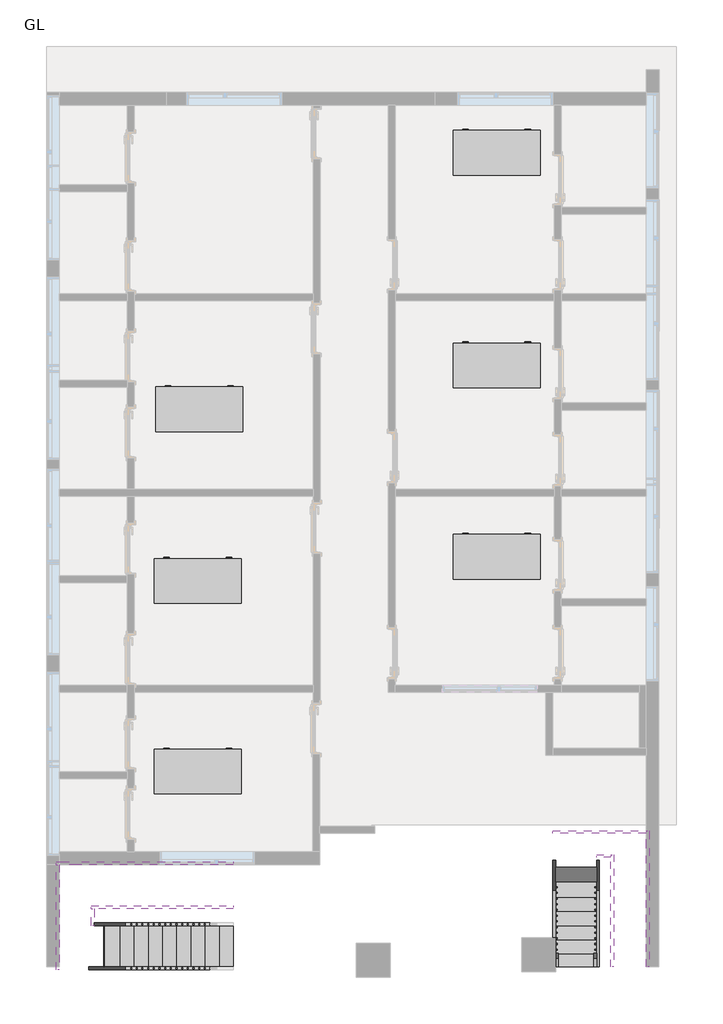
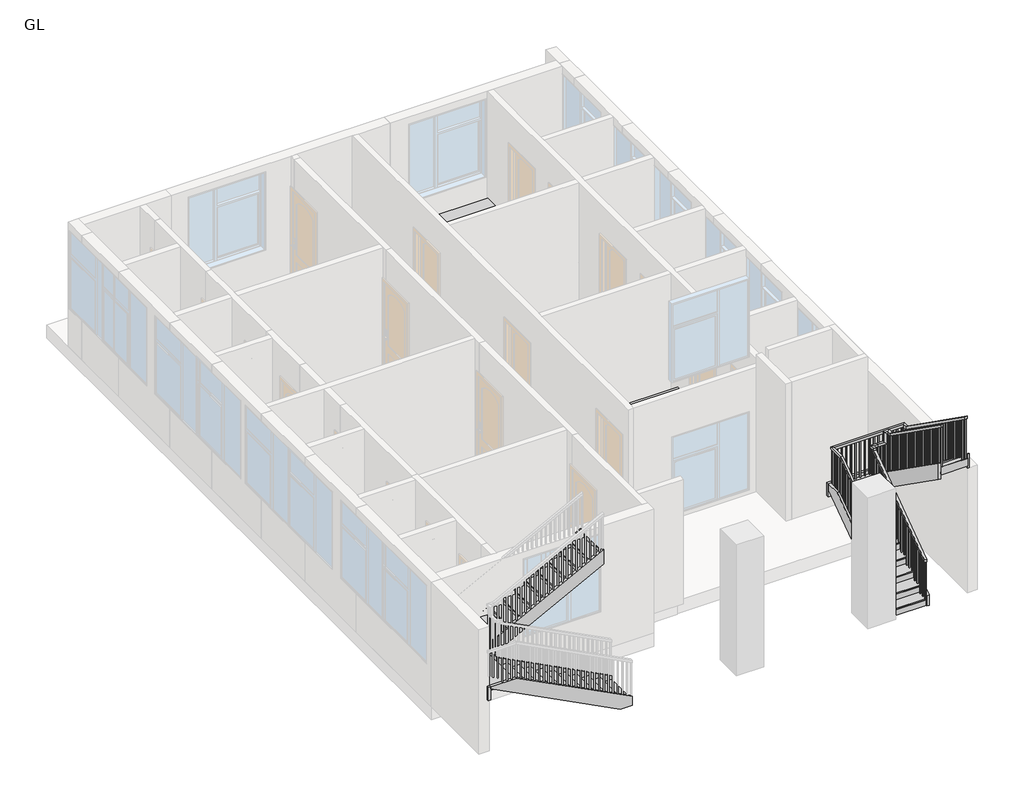
# One storey, part 4 of 4: 12 members, 6 furniture elements, 2 railings, 2 stair flights.
"""IFC4 building model written with IfcOpenShell, lengths in millimetres."""

from ifc_helpers import new_model, si_unit, frame, origin, place, context, project, spatial, polyline, outline, extrude, faceted_brep, transform, mapped, element, save
from components import furniture_072f6425, stair_flight_f3bed003, stair_flight_00806837

model = new_model("IFC4")

# Units and contexts
model_context = context("Model", 3, world=origin())
ifc_project = project(units=[si_unit("LENGTHUNIT", "METRE", prefix="MILLI")], contexts=[model_context])

# Site, building, storey
site = spatial("IfcSite", under=ifc_project)
building = spatial("IfcBuilding", under=site)
storey = spatial("IfcBuildingStorey", under=building, Name="GL", Elevation=0.0)

# Furniture
placement = place(None, origin())
furniture_shape = furniture_072f6425(model_context)
element("IfcFurniture", 1, ObjectType="Desk : 60\" x 30\"", at=placement, inside=storey, context=model_context, shape_type="MappedRepresentation", body=[
    mapped(furniture_shape, transform((-4486.7476406, 1955.9088489, 0.0), x_axis=(1.0, 0.0, 0.0), y_axis=(0.0, 1.0, 0.0), z_axis=(0.0, 0.0, 1.0))),
])
element("IfcFurniture", 2, ObjectType="Desk : 60\" x 30\"", at=placement, inside=storey, context=model_context, shape_type="MappedRepresentation", body=[
    mapped(furniture_shape, transform((-4512.5827262, -1119.7600272, 0.0), x_axis=(1.0, 0.0, 0.0), y_axis=(0.0, 1.0, 0.0), z_axis=(0.0, 0.0, 1.0))),
])
element("IfcFurniture", 3, ObjectType="Desk : 60\" x 30\"", at=placement, inside=storey, context=model_context, shape_type="MappedRepresentation", body=[
    mapped(furniture_shape, transform((839.7412152, -687.9600272, 0.0), x_axis=(1.0, 0.0, 0.0), y_axis=(0.0, 1.0, 0.0), z_axis=(0.0, 0.0, 1.0))),
])
element("IfcFurniture", 4, ObjectType="Desk : 60\" x 30\"", at=placement, inside=storey, context=model_context, shape_type="MappedRepresentation", body=[
    mapped(furniture_shape, transform((839.7412152, 2740.2359967, 0.0), x_axis=(1.0, 0.0, 0.0), y_axis=(0.0, 1.0, 0.0), z_axis=(0.0, 0.0, 1.0))),
])
element("IfcFurniture", 5, ObjectType="Desk : 60\" x 30\"", at=placement, inside=storey, context=model_context, shape_type="MappedRepresentation", body=[
    mapped(furniture_shape, transform((839.7412152, 6551.0399728, 0.0), x_axis=(1.0, 0.0, 0.0), y_axis=(0.0, 1.0, 0.0), z_axis=(0.0, 0.0, 1.0))),
])
element("IfcFurniture", 6, ObjectType="Desk : 60\" x 30\"", at=placement, inside=storey, context=model_context, shape_type="MappedRepresentation", body=[
    mapped(furniture_shape, transform((-4512.5827262, -4536.0600272, 0.0), x_axis=(1.0, 0.0, 0.0), y_axis=(0.0, 1.0, 0.0), z_axis=(0.0, 0.0, 1.0))),
])

# Members
element("IfcMember", 7, ObjectType="Stringer - 2\" Width", at=placement, inside=storey, context=model_context, shape_type="SweptSolid", body=[
    extrude(outline(polyline([(0.0, -3117.2664982), (204.5197081, -3117.2664982), (1524.0, -5663.6319738), (1524.0, -6232.5131972), (1475.4929835, -6232.5131972), (0.0, -3385.0705974), (0.0, -3117.2664982)])), frame((0.0, -7701.7822004, 0.0), z_axis=(0.0, 1.0, 0.0), x_axis=(0.0, 0.0, 1.0)), (0.0, 0.0, 1.0), 50.8),
])
element("IfcMember", 8, ObjectType="Stringer - 2\" Width", at=placement, inside=storey, context=model_context, shape_type="SweptSolid", body=[
    extrude(outline(polyline([(-6232.5131972, -7701.7822004), (-6283.3131972, -7701.7822004), (-6283.3131972, -5824.7082131), (-6232.5131972, -5824.7082131), (-6232.5131972, -7701.7822004)])), frame((0.0, 0.0, 1219.2), z_axis=(0.0, 0.0, 1.0), x_axis=(1.0, 0.0, 0.0)), (0.0, 0.0, 1.0), 304.8),
])
element("IfcMember", 9, ObjectType="Stringer - 2\" Width", at=placement, inside=storey, context=model_context, shape_type="SweptSolid", body=[
    extrude(outline(polyline([(1327.9136913, -6283.3131972), (1219.2, -6283.3131972), (1219.2, -5830.6202937), (2625.2106031, -3117.2664982), (2968.5015263, -3117.2664982), (1327.9136913, -6283.3131972)])), frame((0.0, -5824.7082131, 0.0), z_axis=(0.0, 1.0, 0.0), x_axis=(0.0, 0.0, 1.0)), (0.0, 0.0, 1.0), 50.8),
])
element("IfcMember", 10, ObjectType="Stringer - 2\" Width", at=placement, inside=storey, context=model_context, shape_type="SweptSolid", body=[
    extrude(outline(polyline([(0.0, -3117.2664982), (204.5197081, -3117.2664982), (1494.3778899, -5606.4664982), (1151.0869668, -5606.4664982), (0.0, -3385.0705974), (0.0, -3117.2664982)])), frame((0.0, -6914.3822004, 0.0), z_axis=(0.0, 1.0, 0.0), x_axis=(0.0, 0.0, 1.0)), (0.0, 0.0, 1.0), 50.8),
])
element("IfcMember", 11, ObjectType="Stringer - 2\" Width", at=placement, inside=storey, context=model_context, shape_type="SweptSolid", body=[
    extrude(outline(polyline([(-5606.4664982, -6914.3822004), (-5657.2664982, -6914.3822004), (-5657.2664982, -6609.5822004), (-5606.4664982, -6609.5822004), (-5606.4664982, -6914.3822004)])), frame((0.0, 0.0, 1219.2), z_axis=(0.0, 0.0, 1.0), x_axis=(1.0, 0.0, 0.0)), (0.0, 0.0, 1.0), 304.8),
])
element("IfcMember", 12, ObjectType="Stringer - 2\" Width", at=placement, inside=storey, context=model_context, shape_type="SweptSolid", body=[
    extrude(outline(polyline([(1652.3197081, -5657.2664982), (1309.0287849, -5657.2664982), (2625.2106031, -3117.2664982), (2968.5015263, -3117.2664982), (1652.3197081, -5657.2664982)])), frame((0.0, -6609.5822004, 0.0), z_axis=(0.0, 1.0, 0.0), x_axis=(0.0, 0.0, 1.0)), (0.0, 0.0, 1.0), 50.8),
])
element("IfcMember", 13, ObjectType="Stringer - 2\" Width", at=placement, inside=storey, context=model_context, shape_type="SweptSolid", body=[
    extrude(outline(polyline([(-7650.9822004, 0.0), (-7650.9822004, 239.299187), (-5597.981039, 1676.4), (-5263.3822004, 1676.4), (-5263.3822004, 1538.5633718), (-7461.3298744, 0.0), (-7650.9822004, 0.0)])), frame((2606.6891134, 0.0, 0.0), z_axis=(1.0, 0.0, 0.0), x_axis=(0.0, 1.0, 0.0)), (0.0, 0.0, 1.0), 50.8),
])
element("IfcMember", 14, ObjectType="Stringer - 2\" Width", at=placement, inside=storey, context=model_context, shape_type="SweptSolid", body=[
    extrude(outline(polyline([(2606.6891134, -5263.3822004), (2606.6891134, -5212.5822004), (4281.7311655, -5212.5822004), (4281.7311655, -5263.3822004), (2606.6891134, -5263.3822004)])), frame((0.0, 0.0, 1371.6), z_axis=(0.0, 0.0, 1.0), x_axis=(1.0, 0.0, 0.0)), (0.0, 0.0, 1.0), 304.8),
])
element("IfcMember", 15, ObjectType="Stringer - 2\" Width", at=placement, inside=storey, context=model_context, shape_type="SweptSolid", body=[
    extrude(outline(polyline([(-5212.5822004, 1519.459187), (-5212.5822004, 1371.6), (-5532.8630978, 1371.6), (-7650.9822004, 2854.2833718), (-7650.9822004, 3226.339187), (-5212.5822004, 1519.459187)])), frame((4281.7311655, 0.0, 0.0), z_axis=(1.0, 0.0, 0.0), x_axis=(0.0, 1.0, 0.0)), (0.0, 0.0, 1.0), 50.8),
])
element("IfcMember", 16, ObjectType="Stringer - 2\" Width", at=placement, inside=storey, context=model_context, shape_type="SweptSolid", body=[
    extrude(outline(polyline([(-7650.9822004, 0.0), (-7650.9822004, 239.299187), (-5695.1822004, 1608.359187), (-5695.1822004, 1236.3033718), (-7461.3298744, 0.0), (-7650.9822004, 0.0)])), frame((3394.0891134, 0.0, 0.0), z_axis=(1.0, 0.0, 0.0), x_axis=(0.0, 1.0, 0.0)), (0.0, 0.0, 1.0), 50.8),
])
element("IfcMember", 17, ObjectType="Stringer - 2\" Width", at=placement, inside=storey, context=model_context, shape_type="SweptSolid", body=[
    extrude(outline(polyline([(3394.0891134, -5695.1822004), (3394.0891134, -5644.3822004), (3648.0891134, -5644.3822004), (3648.0891134, -5695.1822004), (3394.0891134, -5695.1822004)])), frame((0.0, 0.0, 1371.6), z_axis=(0.0, 0.0, 1.0), x_axis=(1.0, 0.0, 0.0)), (0.0, 0.0, 1.0), 304.8),
])
element("IfcMember", 18, ObjectType="Stringer - 2\" Width", at=placement, inside=storey, context=model_context, shape_type="SweptSolid", body=[
    extrude(outline(polyline([(-5644.3822004, 1821.719187), (-5644.3822004, 1449.6633718), (-7650.9822004, 2854.2833718), (-7650.9822004, 3226.339187), (-5644.3822004, 1821.719187)])), frame((3648.0891134, 0.0, 0.0), z_axis=(1.0, 0.0, 0.0), x_axis=(0.0, 1.0, 0.0)), (0.0, 0.0, 1.0), 50.8),
])

# Railings
element("IfcRailing", 19, ObjectType="Handrail - Rectangular", at=placement, inside=storey, context=model_context, shape_type="SolidModel", body=[
    faceted_brep([(3343.2891134, -7650.9822004, 1092.2), (3343.2891134, -7650.9822004, 1029.9314749), (3394.0891134, -7650.9822004, 1029.9314749), (3394.0891134, -7650.9822004, 1092.2), (3343.2891134, -5720.5822004, 2460.5848101), (3343.2891134, -5669.7822004, 2434.3264116), (3394.0891134, -5669.7822004, 2434.3264116), (3394.0891134, -5720.5822004, 2460.5848101), (3343.2891134, -5720.5822004, 2514.6), (3343.2891134, -5669.7822004, 2463.8), (3394.0891134, -5669.7822004, 2463.8), (3394.0891134, -5720.5822004, 2514.6), (3343.2891134, -5593.5822004, 2514.6), (3343.2891134, -5593.5822004, 2463.8), (3394.0891134, -5644.3822004, 2463.8), (3394.0891134, -5644.3822004, 2514.6), (3470.2891134, -5593.5822004, 2514.6), (3470.2891134, -5593.5822004, 2463.8), (3470.2891134, -5644.3822004, 2463.8), (3470.2891134, -5644.3822004, 2514.6), (3622.6891134, -5593.5822004, 2514.6), (3673.4891134, -5593.5822004, 2463.8), (3673.4891134, -5644.3822004, 2463.8), (3622.6891134, -5644.3822004, 2514.6), (3622.6891134, -5593.5822004, 2746.4151899), (3673.4891134, -5593.5822004, 2695.6151899), (3673.4891134, -5644.3822004, 2695.6151899), (3622.6891134, -5644.3822004, 2746.4151899), (3749.6891134, -5593.5822004, 2746.4151899), (3749.6891134, -5593.5822004, 2695.6151899), (3698.8891134, -5644.3822004, 2695.6151899), (3698.8891134, -5644.3822004, 2746.4151899), (3749.6891134, -5720.5822004, 2746.4151899), (3749.6891134, -5736.7610126, 2695.6151899), (3698.8891134, -5736.7610126, 2695.6151899), (3698.8891134, -5720.5822004, 2746.4151899), (3749.6891134, -7650.9822004, 4114.8), (3698.8891134, -7650.9822004, 4114.8), (3698.8891134, -7650.9822004, 4052.5314749), (3749.6891134, -7650.9822004, 4052.5314749)], [[[0, 1, 2, 3]], [[1, 0, 4, 5]], [[2, 1, 5, 6]], [[3, 2, 6, 7]], [[0, 3, 7, 4]], [[5, 4, 8, 9]], [[6, 5, 9, 10]], [[7, 6, 10, 11]], [[4, 7, 11, 8]], [[9, 8, 12, 13]], [[10, 9, 13, 14]], [[11, 10, 14, 15]], [[8, 11, 15, 12]], [[13, 12, 16, 17]], [[14, 13, 17, 18]], [[15, 14, 18, 19]], [[12, 15, 19, 16]], [[17, 16, 20, 21]], [[18, 17, 21, 22]], [[19, 18, 22, 23]], [[16, 19, 23, 20]], [[21, 20, 24, 25]], [[22, 21, 25, 26]], [[23, 22, 26, 27]], [[20, 23, 27, 24]], [[25, 24, 28, 29]], [[26, 25, 29, 30]], [[27, 26, 30, 31]], [[24, 27, 31, 28]], [[29, 28, 32, 33]], [[30, 29, 33, 34]], [[31, 30, 34, 35]], [[28, 31, 35, 32]], [[36, 37, 38, 39]], [[33, 32, 36, 39]], [[34, 33, 39, 38]], [[35, 34, 38, 37]], [[32, 35, 37, 36]]]),
    extrude(outline(polyline([(-7558.9072004, 3987.2631205), (-7539.8572004, 3973.759323), (-7539.8572004, 3022.6), (-7558.9072004, 3022.6), (-7558.9072004, 3987.2631205)])), frame((3714.7641134, 0.0, 0.0), z_axis=(1.0, 0.0, 0.0), x_axis=(0.0, 1.0, 0.0)), (0.0, 0.0, 1.0), 19.05),
    extrude(outline(polyline([(-7457.3072004, 3915.2428673), (-7438.2572004, 3901.7390699), (-7438.2572004, 3022.6), (-7457.3072004, 3022.6), (-7457.3072004, 3915.2428673)])), frame((3714.7641134, 0.0, 0.0), z_axis=(1.0, 0.0, 0.0), x_axis=(0.0, 1.0, 0.0)), (0.0, 0.0, 1.0), 19.05),
    extrude(outline(polyline([(-7355.7072004, 3843.2226142), (-7336.6572004, 3829.7188167), (-7336.6572004, 2844.8), (-7355.7072004, 2844.8), (-7355.7072004, 3843.2226142)])), frame((3714.7641134, 0.0, 0.0), z_axis=(1.0, 0.0, 0.0), x_axis=(0.0, 1.0, 0.0)), (0.0, 0.0, 1.0), 19.05),
    extrude(outline(polyline([(-7254.1072004, 3771.202361), (-7235.0572004, 3757.6985635), (-7235.0572004, 2844.8), (-7254.1072004, 2844.8), (-7254.1072004, 3771.202361)])), frame((3714.7641134, 0.0, 0.0), z_axis=(1.0, 0.0, 0.0), x_axis=(0.0, 1.0, 0.0)), (0.0, 0.0, 1.0), 19.05),
    extrude(outline(polyline([(-7152.5072004, 3699.1821078), (-7133.4572004, 3685.6783104), (-7133.4572004, 2667.0), (-7152.5072004, 2667.0), (-7152.5072004, 3699.1821078)])), frame((3714.7641134, 0.0, 0.0), z_axis=(1.0, 0.0, 0.0), x_axis=(0.0, 1.0, 0.0)), (0.0, 0.0, 1.0), 19.05),
    extrude(outline(polyline([(-7050.9072004, 3627.1618547), (-7031.8572004, 3613.6580572), (-7031.8572004, 2667.0), (-7050.9072004, 2667.0), (-7050.9072004, 3627.1618547)])), frame((3714.7641134, 0.0, 0.0), z_axis=(1.0, 0.0, 0.0), x_axis=(0.0, 1.0, 0.0)), (0.0, 0.0, 1.0), 19.05),
    extrude(outline(polyline([(-6949.3072004, 3555.1416015), (-6930.2572004, 3541.637804), (-6930.2572004, 2667.0), (-6949.3072004, 2667.0), (-6949.3072004, 3555.1416015)])), frame((3714.7641134, 0.0, 0.0), z_axis=(1.0, 0.0, 0.0), x_axis=(0.0, 1.0, 0.0)), (0.0, 0.0, 1.0), 19.05),
    extrude(outline(polyline([(-6847.7072004, 3483.1213483), (-6828.6572004, 3469.6175509), (-6828.6572004, 2489.2), (-6847.7072004, 2489.2), (-6847.7072004, 3483.1213483)])), frame((3714.7641134, 0.0, 0.0), z_axis=(1.0, 0.0, 0.0), x_axis=(0.0, 1.0, 0.0)), (0.0, 0.0, 1.0), 19.05),
    extrude(outline(polyline([(-6746.1072004, 3411.1010952), (-6727.0572004, 3397.5972977), (-6727.0572004, 2489.2), (-6746.1072004, 2489.2), (-6746.1072004, 3411.1010952)])), frame((3714.7641134, 0.0, 0.0), z_axis=(1.0, 0.0, 0.0), x_axis=(0.0, 1.0, 0.0)), (0.0, 0.0, 1.0), 19.05),
    extrude(outline(polyline([(-6644.5072004, 3339.080842), (-6625.4572004, 3325.5770445), (-6625.4572004, 2311.4), (-6644.5072004, 2311.4), (-6644.5072004, 3339.080842)])), frame((3714.7641134, 0.0, 0.0), z_axis=(1.0, 0.0, 0.0), x_axis=(0.0, 1.0, 0.0)), (0.0, 0.0, 1.0), 19.05),
    extrude(outline(polyline([(-6542.9072004, 3267.0605888), (-6523.8572004, 3253.5567914), (-6523.8572004, 2311.4), (-6542.9072004, 2311.4), (-6542.9072004, 3267.0605888)])), frame((3714.7641134, 0.0, 0.0), z_axis=(1.0, 0.0, 0.0), x_axis=(0.0, 1.0, 0.0)), (0.0, 0.0, 1.0), 19.05),
    extrude(outline(polyline([(-6441.3072004, 3195.0403357), (-6422.2572004, 3181.5365382), (-6422.2572004, 2311.4), (-6441.3072004, 2311.4), (-6441.3072004, 3195.0403357)])), frame((3714.7641134, 0.0, 0.0), z_axis=(1.0, 0.0, 0.0), x_axis=(0.0, 1.0, 0.0)), (0.0, 0.0, 1.0), 19.05),
    extrude(outline(polyline([(-6339.7072004, 3123.0200825), (-6320.6572004, 3109.516285), (-6320.6572004, 2133.6), (-6339.7072004, 2133.6), (-6339.7072004, 3123.0200825)])), frame((3714.7641134, 0.0, 0.0), z_axis=(1.0, 0.0, 0.0), x_axis=(0.0, 1.0, 0.0)), (0.0, 0.0, 1.0), 19.05),
    extrude(outline(polyline([(-6238.1072004, 3050.9998293), (-6219.0572004, 3037.4960319), (-6219.0572004, 2133.6), (-6238.1072004, 2133.6), (-6238.1072004, 3050.9998293)])), frame((3714.7641134, 0.0, 0.0), z_axis=(1.0, 0.0, 0.0), x_axis=(0.0, 1.0, 0.0)), (0.0, 0.0, 1.0), 19.05),
    extrude(outline(polyline([(-6136.5072004, 2978.9795762), (-6117.4572004, 2965.4757787), (-6117.4572004, 1955.8), (-6136.5072004, 1955.8), (-6136.5072004, 2978.9795762)])), frame((3714.7641134, 0.0, 0.0), z_axis=(1.0, 0.0, 0.0), x_axis=(0.0, 1.0, 0.0)), (0.0, 0.0, 1.0), 19.05),
    extrude(outline(polyline([(-6034.9072004, 2906.959323), (-6015.8572004, 2893.4555255), (-6015.8572004, 1955.8), (-6034.9072004, 1955.8), (-6034.9072004, 2906.959323)])), frame((3714.7641134, 0.0, 0.0), z_axis=(1.0, 0.0, 0.0), x_axis=(0.0, 1.0, 0.0)), (0.0, 0.0, 1.0), 19.05),
    extrude(outline(polyline([(-5933.3072004, 2834.9390699), (-5914.2572004, 2821.4352724), (-5914.2572004, 1955.8), (-5933.3072004, 1955.8), (-5933.3072004, 2834.9390699)])), frame((3714.7641134, 0.0, 0.0), z_axis=(1.0, 0.0, 0.0), x_axis=(0.0, 1.0, 0.0)), (0.0, 0.0, 1.0), 19.05),
    extrude(outline(polyline([(-5831.7072004, 2762.9188167), (-5812.6572004, 2749.4150192), (-5812.6572004, 1778.0), (-5831.7072004, 1778.0), (-5831.7072004, 2762.9188167)])), frame((3714.7641134, 0.0, 0.0), z_axis=(1.0, 0.0, 0.0), x_axis=(0.0, 1.0, 0.0)), (0.0, 0.0, 1.0), 19.05),
    extrude(outline(polyline([(-5730.1072004, 2690.8985635), (-5711.0572004, 2677.3947661), (-5711.0572004, 1778.0), (-5730.1072004, 1778.0), (-5730.1072004, 2690.8985635)])), frame((3714.7641134, 0.0, 0.0), z_axis=(1.0, 0.0, 0.0), x_axis=(0.0, 1.0, 0.0)), (0.0, 0.0, 1.0), 19.05),
    extrude(outline(polyline([(3663.9641134, -5628.5072004), (3663.9641134, -5609.4572004), (3683.0141134, -5609.4572004), (3683.0141134, -5628.5072004), (3663.9641134, -5628.5072004)])), frame((0.0, 0.0, 1600.2), z_axis=(0.0, 0.0, 1.0), x_axis=(1.0, 0.0, 0.0)), (0.0, 0.0, 1.0), 1095.4151899),
    extrude(outline(polyline([(3562.3641134, -5628.5072004), (3562.3641134, -5609.4572004), (3581.4141134, -5609.4572004), (3581.4141134, -5628.5072004), (3562.3641134, -5628.5072004)])), frame((0.0, 0.0, 1600.2), z_axis=(0.0, 0.0, 1.0), x_axis=(1.0, 0.0, 0.0)), (0.0, 0.0, 1.0), 863.6),
    extrude(outline(polyline([(3460.7641134, -5628.5072004), (3460.7641134, -5609.4572004), (3479.8141134, -5609.4572004), (3479.8141134, -5628.5072004), (3460.7641134, -5628.5072004)])), frame((0.0, 0.0, 1600.2), z_axis=(0.0, 0.0, 1.0), x_axis=(1.0, 0.0, 0.0)), (0.0, 0.0, 1.0), 863.6),
    extrude(outline(polyline([(-5730.1072004, 2391.5643863), (-5711.0572004, 2405.0681838), (-5711.0572004, 1422.4), (-5730.1072004, 1422.4), (-5730.1072004, 2391.5643863)])), frame((3359.1641134, 0.0, 0.0), z_axis=(1.0, 0.0, 0.0), x_axis=(0.0, 1.0, 0.0)), (0.0, 0.0, 1.0), 19.05),
    extrude(outline(polyline([(-5831.7072004, 2319.5441331), (-5812.6572004, 2333.0479306), (-5812.6572004, 1422.4), (-5831.7072004, 1422.4), (-5831.7072004, 2319.5441331)])), frame((3359.1641134, 0.0, 0.0), z_axis=(1.0, 0.0, 0.0), x_axis=(0.0, 1.0, 0.0)), (0.0, 0.0, 1.0), 19.05),
    extrude(outline(polyline([(-5933.3072004, 2247.52388), (-5914.2572004, 2261.0276774), (-5914.2572004, 1244.6), (-5933.3072004, 1244.6), (-5933.3072004, 2247.52388)])), frame((3359.1641134, 0.0, 0.0), z_axis=(1.0, 0.0, 0.0), x_axis=(0.0, 1.0, 0.0)), (0.0, 0.0, 1.0), 19.05),
    extrude(outline(polyline([(-6034.9072004, 2175.5036268), (-6015.8572004, 2189.0074243), (-6015.8572004, 1244.6), (-6034.9072004, 1244.6), (-6034.9072004, 2175.5036268)])), frame((3359.1641134, 0.0, 0.0), z_axis=(1.0, 0.0, 0.0), x_axis=(0.0, 1.0, 0.0)), (0.0, 0.0, 1.0), 19.05),
    extrude(outline(polyline([(-6136.5072004, 2103.4833736), (-6117.4572004, 2116.9871711), (-6117.4572004, 1244.6), (-6136.5072004, 1244.6), (-6136.5072004, 2103.4833736)])), frame((3359.1641134, 0.0, 0.0), z_axis=(1.0, 0.0, 0.0), x_axis=(0.0, 1.0, 0.0)), (0.0, 0.0, 1.0), 19.05),
    extrude(outline(polyline([(-6238.1072004, 2031.4631205), (-6219.0572004, 2044.966918), (-6219.0572004, 1066.8), (-6238.1072004, 1066.8), (-6238.1072004, 2031.4631205)])), frame((3359.1641134, 0.0, 0.0), z_axis=(1.0, 0.0, 0.0), x_axis=(0.0, 1.0, 0.0)), (0.0, 0.0, 1.0), 19.05),
    extrude(outline(polyline([(-6339.7072004, 1959.4428673), (-6320.6572004, 1972.9466648), (-6320.6572004, 1066.8), (-6339.7072004, 1066.8), (-6339.7072004, 1959.4428673)])), frame((3359.1641134, 0.0, 0.0), z_axis=(1.0, 0.0, 0.0), x_axis=(0.0, 1.0, 0.0)), (0.0, 0.0, 1.0), 19.05),
    extrude(outline(polyline([(-6441.3072004, 1887.4226142), (-6422.2572004, 1900.9264116), (-6422.2572004, 889.0), (-6441.3072004, 889.0), (-6441.3072004, 1887.4226142)])), frame((3359.1641134, 0.0, 0.0), z_axis=(1.0, 0.0, 0.0), x_axis=(0.0, 1.0, 0.0)), (0.0, 0.0, 1.0), 19.05),
    extrude(outline(polyline([(-6542.9072004, 1815.402361), (-6523.8572004, 1828.9061585), (-6523.8572004, 889.0), (-6542.9072004, 889.0), (-6542.9072004, 1815.402361)])), frame((3359.1641134, 0.0, 0.0), z_axis=(1.0, 0.0, 0.0), x_axis=(0.0, 1.0, 0.0)), (0.0, 0.0, 1.0), 19.05),
    extrude(outline(polyline([(-6644.5072004, 1743.3821078), (-6625.4572004, 1756.8859053), (-6625.4572004, 889.0), (-6644.5072004, 889.0), (-6644.5072004, 1743.3821078)])), frame((3359.1641134, 0.0, 0.0), z_axis=(1.0, 0.0, 0.0), x_axis=(0.0, 1.0, 0.0)), (0.0, 0.0, 1.0), 19.05),
    extrude(outline(polyline([(-6746.1072004, 1671.3618547), (-6727.0572004, 1684.8656521), (-6727.0572004, 711.2), (-6746.1072004, 711.2), (-6746.1072004, 1671.3618547)])), frame((3359.1641134, 0.0, 0.0), z_axis=(1.0, 0.0, 0.0), x_axis=(0.0, 1.0, 0.0)), (0.0, 0.0, 1.0), 19.05),
    extrude(outline(polyline([(-6847.7072004, 1599.3416015), (-6828.6572004, 1612.845399), (-6828.6572004, 711.2), (-6847.7072004, 711.2), (-6847.7072004, 1599.3416015)])), frame((3359.1641134, 0.0, 0.0), z_axis=(1.0, 0.0, 0.0), x_axis=(0.0, 1.0, 0.0)), (0.0, 0.0, 1.0), 19.05),
    extrude(outline(polyline([(-6949.3072004, 1527.3213483), (-6930.2572004, 1540.8251458), (-6930.2572004, 533.4), (-6949.3072004, 533.4), (-6949.3072004, 1527.3213483)])), frame((3359.1641134, 0.0, 0.0), z_axis=(1.0, 0.0, 0.0), x_axis=(0.0, 1.0, 0.0)), (0.0, 0.0, 1.0), 19.05),
    extrude(outline(polyline([(-7050.9072004, 1455.3010952), (-7031.8572004, 1468.8048926), (-7031.8572004, 533.4), (-7050.9072004, 533.4), (-7050.9072004, 1455.3010952)])), frame((3359.1641134, 0.0, 0.0), z_axis=(1.0, 0.0, 0.0), x_axis=(0.0, 1.0, 0.0)), (0.0, 0.0, 1.0), 19.05),
    extrude(outline(polyline([(-7152.5072004, 1383.280842), (-7133.4572004, 1396.7846395), (-7133.4572004, 533.4), (-7152.5072004, 533.4), (-7152.5072004, 1383.280842)])), frame((3359.1641134, 0.0, 0.0), z_axis=(1.0, 0.0, 0.0), x_axis=(0.0, 1.0, 0.0)), (0.0, 0.0, 1.0), 19.05),
    extrude(outline(polyline([(-7254.1072004, 1311.2605888), (-7235.0572004, 1324.7643863), (-7235.0572004, 355.6), (-7254.1072004, 355.6), (-7254.1072004, 1311.2605888)])), frame((3359.1641134, 0.0, 0.0), z_axis=(1.0, 0.0, 0.0), x_axis=(0.0, 1.0, 0.0)), (0.0, 0.0, 1.0), 19.05),
    extrude(outline(polyline([(-7355.7072004, 1239.2403357), (-7336.6572004, 1252.7441331), (-7336.6572004, 355.6), (-7355.7072004, 355.6), (-7355.7072004, 1239.2403357)])), frame((3359.1641134, 0.0, 0.0), z_axis=(1.0, 0.0, 0.0), x_axis=(0.0, 1.0, 0.0)), (0.0, 0.0, 1.0), 19.05),
    extrude(outline(polyline([(-7457.3072004, 1167.2200825), (-7438.2572004, 1180.72388), (-7438.2572004, 177.8), (-7457.3072004, 177.8), (-7457.3072004, 1167.2200825)])), frame((3359.1641134, 0.0, 0.0), z_axis=(1.0, 0.0, 0.0), x_axis=(0.0, 1.0, 0.0)), (0.0, 0.0, 1.0), 19.05),
    extrude(outline(polyline([(-7558.9072004, 1095.1998293), (-7539.8572004, 1108.7036268), (-7539.8572004, 177.8), (-7558.9072004, 177.8), (-7558.9072004, 1095.1998293)])), frame((3359.1641134, 0.0, 0.0), z_axis=(1.0, 0.0, 0.0), x_axis=(0.0, 1.0, 0.0)), (0.0, 0.0, 1.0), 19.05),
    extrude(outline(polyline([(3714.7641134, -5628.5072004), (3714.7641134, -5609.4572004), (3733.8141134, -5609.4572004), (3733.8141134, -5628.5072004), (3714.7641134, -5628.5072004)])), frame((0.0, 0.0, 1600.2), z_axis=(0.0, 0.0, 1.0), x_axis=(1.0, 0.0, 0.0)), (0.0, 0.0, 1.0), 1095.4151899),
    extrude(outline(polyline([(3378.2141134, -5628.5072004), (3359.1641134, -5628.5072004), (3359.1641134, -5609.4572004), (3378.2141134, -5609.4572004), (3378.2141134, -5628.5072004)])), frame((0.0, 0.0, 1600.2), z_axis=(0.0, 0.0, 1.0), x_axis=(1.0, 0.0, 0.0)), (0.0, 0.0, 1.0), 863.6),
    extrude(outline(polyline([(-7650.9822004, 4052.5314749), (-7631.9322004, 4039.0276774), (-7631.9322004, 3022.6), (-7650.9822004, 3022.6), (-7650.9822004, 4052.5314749)])), frame((3714.7641134, 0.0, 0.0), z_axis=(1.0, 0.0, 0.0), x_axis=(0.0, 1.0, 0.0)), (0.0, 0.0, 1.0), 19.05),
    extrude(outline(polyline([(-7650.9822004, 1029.9314749), (-7631.9322004, 1043.4352724), (-7631.9322004, 177.8), (-7650.9822004, 177.8), (-7650.9822004, 1029.9314749)])), frame((3359.1641134, 0.0, 0.0), z_axis=(1.0, 0.0, 0.0), x_axis=(0.0, 1.0, 0.0)), (0.0, 0.0, 1.0), 19.05),
])
element("IfcRailing", 20, ObjectType="Handrail - Rectangular", at=placement, inside=storey, context=model_context, shape_type="SolidModel", body=[
    faceted_brep([(2657.4891134, -7650.9822004, 1092.2), (2657.4891134, -7650.9822004, 1029.9314749), (2708.2891134, -7650.9822004, 1029.9314749), (2708.2891134, -7650.9822004, 1092.2), (2657.4891134, -5644.3822004, 2514.6), (2657.4891134, -5628.2033882, 2463.8), (2708.2891134, -5628.2033882, 2463.8), (2708.2891134, -5644.3822004, 2514.6), (2657.4891134, -5263.3822004, 2514.6), (2657.4891134, -5263.3822004, 2463.8), (2708.2891134, -5314.1822004, 2463.8), (2708.2891134, -5314.1822004, 2514.6), (4281.7311655, -5263.3822004, 2514.6), (4281.7311655, -5263.3822004, 2463.8), (4230.9311655, -5314.1822004, 2463.8), (4230.9311655, -5314.1822004, 2514.6), (4281.7311655, -5393.5572004, 2514.6), (4281.7311655, -5409.7360126, 2463.8), (4230.9311655, -5409.7360126, 2463.8), (4230.9311655, -5393.5572004, 2514.6), (4281.7311655, -7650.9822004, 4114.8), (4230.9311655, -7650.9822004, 4114.8), (4230.9311655, -7650.9822004, 4052.5314749), (4281.7311655, -7650.9822004, 4052.5314749)], [[[0, 1, 2, 3]], [[1, 0, 4, 5]], [[2, 1, 5, 6]], [[3, 2, 6, 7]], [[0, 3, 7, 4]], [[5, 4, 8, 9]], [[6, 5, 9, 10]], [[7, 6, 10, 11]], [[4, 7, 11, 8]], [[9, 8, 12, 13]], [[10, 9, 13, 14]], [[11, 10, 14, 15]], [[8, 11, 15, 12]], [[13, 12, 16, 17]], [[14, 13, 17, 18]], [[15, 14, 18, 19]], [[12, 15, 19, 16]], [[20, 21, 22, 23]], [[17, 16, 20, 23]], [[18, 17, 23, 22]], [[19, 18, 22, 21]], [[16, 19, 21, 20]]]),
    extrude(outline(polyline([(-7616.0572004, 4027.7745129), (-7616.0572004, 3022.6), (-7635.1072004, 3022.6), (-7635.1072004, 4041.2783104), (-7616.0572004, 4027.7745129)])), frame((4246.8061655, 0.0, 0.0), z_axis=(1.0, 0.0, 0.0), x_axis=(0.0, 1.0, 0.0)), (0.0, 0.0, 1.0), 19.05),
    extrude(outline(polyline([(-7514.4572004, 3955.7542597), (-7514.4572004, 3022.6), (-7533.5072004, 3022.6), (-7533.5072004, 3969.2580572), (-7514.4572004, 3955.7542597)])), frame((4246.8061655, 0.0, 0.0), z_axis=(1.0, 0.0, 0.0), x_axis=(0.0, 1.0, 0.0)), (0.0, 0.0, 1.0), 19.05),
    extrude(outline(polyline([(-7412.8572004, 3883.7340066), (-7412.8572004, 3022.6), (-7431.9072004, 3022.6), (-7431.9072004, 3897.237804), (-7412.8572004, 3883.7340066)])), frame((4246.8061655, 0.0, 0.0), z_axis=(1.0, 0.0, 0.0), x_axis=(0.0, 1.0, 0.0)), (0.0, 0.0, 1.0), 19.05),
    extrude(outline(polyline([(-7311.2572004, 3811.7137534), (-7311.2572004, 2844.8), (-7330.3072004, 2844.8), (-7330.3072004, 3825.2175509), (-7311.2572004, 3811.7137534)])), frame((4246.8061655, 0.0, 0.0), z_axis=(1.0, 0.0, 0.0), x_axis=(0.0, 1.0, 0.0)), (0.0, 0.0, 1.0), 19.05),
    extrude(outline(polyline([(-7209.6572004, 3739.6935002), (-7209.6572004, 2844.8), (-7228.7072004, 2844.8), (-7228.7072004, 3753.1972977), (-7209.6572004, 3739.6935002)])), frame((4246.8061655, 0.0, 0.0), z_axis=(1.0, 0.0, 0.0), x_axis=(0.0, 1.0, 0.0)), (0.0, 0.0, 1.0), 19.05),
    extrude(outline(polyline([(-7108.0572004, 3667.6732471), (-7108.0572004, 2667.0), (-7127.1072004, 2667.0), (-7127.1072004, 3681.1770445), (-7108.0572004, 3667.6732471)])), frame((4246.8061655, 0.0, 0.0), z_axis=(1.0, 0.0, 0.0), x_axis=(0.0, 1.0, 0.0)), (0.0, 0.0, 1.0), 19.05),
    extrude(outline(polyline([(-7006.4572004, 3595.6529939), (-7006.4572004, 2667.0), (-7025.5072004, 2667.0), (-7025.5072004, 3609.1567914), (-7006.4572004, 3595.6529939)])), frame((4246.8061655, 0.0, 0.0), z_axis=(1.0, 0.0, 0.0), x_axis=(0.0, 1.0, 0.0)), (0.0, 0.0, 1.0), 19.05),
    extrude(outline(polyline([(-6904.8572004, 3523.6327407), (-6904.8572004, 2667.0), (-6923.9072004, 2667.0), (-6923.9072004, 3537.1365382), (-6904.8572004, 3523.6327407)])), frame((4246.8061655, 0.0, 0.0), z_axis=(1.0, 0.0, 0.0), x_axis=(0.0, 1.0, 0.0)), (0.0, 0.0, 1.0), 19.05),
    extrude(outline(polyline([(-6803.2572004, 3451.6124876), (-6803.2572004, 2489.2), (-6822.3072004, 2489.2), (-6822.3072004, 3465.116285), (-6803.2572004, 3451.6124876)])), frame((4246.8061655, 0.0, 0.0), z_axis=(1.0, 0.0, 0.0), x_axis=(0.0, 1.0, 0.0)), (0.0, 0.0, 1.0), 19.05),
    extrude(outline(polyline([(-6701.6572004, 3379.5922344), (-6701.6572004, 2489.2), (-6720.7072004, 2489.2), (-6720.7072004, 3393.0960319), (-6701.6572004, 3379.5922344)])), frame((4246.8061655, 0.0, 0.0), z_axis=(1.0, 0.0, 0.0), x_axis=(0.0, 1.0, 0.0)), (0.0, 0.0, 1.0), 19.05),
    extrude(outline(polyline([(-6600.0572004, 3307.5719812), (-6600.0572004, 2311.4), (-6619.1072004, 2311.4), (-6619.1072004, 3321.0757787), (-6600.0572004, 3307.5719812)])), frame((4246.8061655, 0.0, 0.0), z_axis=(1.0, 0.0, 0.0), x_axis=(0.0, 1.0, 0.0)), (0.0, 0.0, 1.0), 19.05),
    extrude(outline(polyline([(-6498.4572004, 3235.5517281), (-6498.4572004, 2311.4), (-6517.5072004, 2311.4), (-6517.5072004, 3249.0555255), (-6498.4572004, 3235.5517281)])), frame((4246.8061655, 0.0, 0.0), z_axis=(1.0, 0.0, 0.0), x_axis=(0.0, 1.0, 0.0)), (0.0, 0.0, 1.0), 19.05),
    extrude(outline(polyline([(-6396.8572004, 3163.5314749), (-6396.8572004, 2311.4), (-6415.9072004, 2311.4), (-6415.9072004, 3177.0352724), (-6396.8572004, 3163.5314749)])), frame((4246.8061655, 0.0, 0.0), z_axis=(1.0, 0.0, 0.0), x_axis=(0.0, 1.0, 0.0)), (0.0, 0.0, 1.0), 19.05),
    extrude(outline(polyline([(-6295.2572004, 3091.5112217), (-6295.2572004, 2133.6), (-6314.3072004, 2133.6), (-6314.3072004, 3105.0150192), (-6295.2572004, 3091.5112217)])), frame((4246.8061655, 0.0, 0.0), z_axis=(1.0, 0.0, 0.0), x_axis=(0.0, 1.0, 0.0)), (0.0, 0.0, 1.0), 19.05),
    extrude(outline(polyline([(-6193.6572004, 3019.4909686), (-6193.6572004, 2133.6), (-6212.7072004, 2133.6), (-6212.7072004, 3032.9947661), (-6193.6572004, 3019.4909686)])), frame((4246.8061655, 0.0, 0.0), z_axis=(1.0, 0.0, 0.0), x_axis=(0.0, 1.0, 0.0)), (0.0, 0.0, 1.0), 19.05),
    extrude(outline(polyline([(-6092.0572004, 2947.4707154), (-6092.0572004, 1955.8), (-6111.1072004, 1955.8), (-6111.1072004, 2960.9745129), (-6092.0572004, 2947.4707154)])), frame((4246.8061655, 0.0, 0.0), z_axis=(1.0, 0.0, 0.0), x_axis=(0.0, 1.0, 0.0)), (0.0, 0.0, 1.0), 19.05),
    extrude(outline(polyline([(-5990.4572004, 2875.4504623), (-5990.4572004, 1955.8), (-6009.5072004, 1955.8), (-6009.5072004, 2888.9542597), (-5990.4572004, 2875.4504623)])), frame((4246.8061655, 0.0, 0.0), z_axis=(1.0, 0.0, 0.0), x_axis=(0.0, 1.0, 0.0)), (0.0, 0.0, 1.0), 19.05),
    extrude(outline(polyline([(-5888.8572004, 2803.4302091), (-5888.8572004, 1955.8), (-5907.9072004, 1955.8), (-5907.9072004, 2816.9340066), (-5888.8572004, 2803.4302091)])), frame((4246.8061655, 0.0, 0.0), z_axis=(1.0, 0.0, 0.0), x_axis=(0.0, 1.0, 0.0)), (0.0, 0.0, 1.0), 19.05),
    extrude(outline(polyline([(-5787.2572004, 2731.4099559), (-5787.2572004, 1778.0), (-5806.3072004, 1778.0), (-5806.3072004, 2744.9137534), (-5787.2572004, 2731.4099559)])), frame((4246.8061655, 0.0, 0.0), z_axis=(1.0, 0.0, 0.0), x_axis=(0.0, 1.0, 0.0)), (0.0, 0.0, 1.0), 19.05),
    extrude(outline(polyline([(-5685.6572004, 2659.3897028), (-5685.6572004, 1778.0), (-5704.7072004, 1778.0), (-5704.7072004, 2672.8935002), (-5685.6572004, 2659.3897028)])), frame((4246.8061655, 0.0, 0.0), z_axis=(1.0, 0.0, 0.0), x_axis=(0.0, 1.0, 0.0)), (0.0, 0.0, 1.0), 19.05),
    extrude(outline(polyline([(-5584.0572004, 2587.3694496), (-5584.0572004, 1600.2), (-5603.1072004, 1600.2), (-5603.1072004, 2600.8732471), (-5584.0572004, 2587.3694496)])), frame((4246.8061655, 0.0, 0.0), z_axis=(1.0, 0.0, 0.0), x_axis=(0.0, 1.0, 0.0)), (0.0, 0.0, 1.0), 19.05),
    extrude(outline(polyline([(-5482.4572004, 2515.3491964), (-5482.4572004, 1600.2), (-5501.5072004, 1600.2), (-5501.5072004, 2528.8529939), (-5482.4572004, 2515.3491964)])), frame((4246.8061655, 0.0, 0.0), z_axis=(1.0, 0.0, 0.0), x_axis=(0.0, 1.0, 0.0)), (0.0, 0.0, 1.0), 19.05),
    extrude(outline(polyline([(4265.8561655, -5380.8572004), (4265.8561655, -5399.9072004), (4246.8061655, -5399.9072004), (4246.8061655, -5380.8572004), (4265.8561655, -5380.8572004)])), frame((0.0, 0.0, 1600.2), z_axis=(0.0, 0.0, 1.0), x_axis=(1.0, 0.0, 0.0)), (0.0, 0.0, 1.0), 863.6),
    extrude(outline(polyline([(4197.3641134, -5279.2572004), (4216.4141134, -5279.2572004), (4216.4141134, -5298.3072004), (4197.3641134, -5298.3072004), (4197.3641134, -5279.2572004)])), frame((0.0, 0.0, 1600.2), z_axis=(0.0, 0.0, 1.0), x_axis=(1.0, 0.0, 0.0)), (0.0, 0.0, 1.0), 863.6),
    extrude(outline(polyline([(4095.7641134, -5279.2572004), (4114.8141134, -5279.2572004), (4114.8141134, -5298.3072004), (4095.7641134, -5298.3072004), (4095.7641134, -5279.2572004)])), frame((0.0, 0.0, 1600.2), z_axis=(0.0, 0.0, 1.0), x_axis=(1.0, 0.0, 0.0)), (0.0, 0.0, 1.0), 863.6),
    extrude(outline(polyline([(3994.1641134, -5279.2572004), (4013.2141134, -5279.2572004), (4013.2141134, -5298.3072004), (3994.1641134, -5298.3072004), (3994.1641134, -5279.2572004)])), frame((0.0, 0.0, 1600.2), z_axis=(0.0, 0.0, 1.0), x_axis=(1.0, 0.0, 0.0)), (0.0, 0.0, 1.0), 863.6),
    extrude(outline(polyline([(3892.5641134, -5279.2572004), (3911.6141134, -5279.2572004), (3911.6141134, -5298.3072004), (3892.5641134, -5298.3072004), (3892.5641134, -5279.2572004)])), frame((0.0, 0.0, 1600.2), z_axis=(0.0, 0.0, 1.0), x_axis=(1.0, 0.0, 0.0)), (0.0, 0.0, 1.0), 863.6),
    extrude(outline(polyline([(3790.9641134, -5279.2572004), (3810.0141134, -5279.2572004), (3810.0141134, -5298.3072004), (3790.9641134, -5298.3072004), (3790.9641134, -5279.2572004)])), frame((0.0, 0.0, 1600.2), z_axis=(0.0, 0.0, 1.0), x_axis=(1.0, 0.0, 0.0)), (0.0, 0.0, 1.0), 863.6),
    extrude(outline(polyline([(3689.3641134, -5279.2572004), (3708.4141134, -5279.2572004), (3708.4141134, -5298.3072004), (3689.3641134, -5298.3072004), (3689.3641134, -5279.2572004)])), frame((0.0, 0.0, 1600.2), z_axis=(0.0, 0.0, 1.0), x_axis=(1.0, 0.0, 0.0)), (0.0, 0.0, 1.0), 863.6),
    extrude(outline(polyline([(3587.7641134, -5279.2572004), (3606.8141134, -5279.2572004), (3606.8141134, -5298.3072004), (3587.7641134, -5298.3072004), (3587.7641134, -5279.2572004)])), frame((0.0, 0.0, 1600.2), z_axis=(0.0, 0.0, 1.0), x_axis=(1.0, 0.0, 0.0)), (0.0, 0.0, 1.0), 863.6),
    extrude(outline(polyline([(3486.1641134, -5279.2572004), (3505.2141134, -5279.2572004), (3505.2141134, -5298.3072004), (3486.1641134, -5298.3072004), (3486.1641134, -5279.2572004)])), frame((0.0, 0.0, 1600.2), z_axis=(0.0, 0.0, 1.0), x_axis=(1.0, 0.0, 0.0)), (0.0, 0.0, 1.0), 863.6),
    extrude(outline(polyline([(3384.5641134, -5279.2572004), (3403.6141134, -5279.2572004), (3403.6141134, -5298.3072004), (3384.5641134, -5298.3072004), (3384.5641134, -5279.2572004)])), frame((0.0, 0.0, 1600.2), z_axis=(0.0, 0.0, 1.0), x_axis=(1.0, 0.0, 0.0)), (0.0, 0.0, 1.0), 863.6),
    extrude(outline(polyline([(3282.9641134, -5279.2572004), (3302.0141134, -5279.2572004), (3302.0141134, -5298.3072004), (3282.9641134, -5298.3072004), (3282.9641134, -5279.2572004)])), frame((0.0, 0.0, 1600.2), z_axis=(0.0, 0.0, 1.0), x_axis=(1.0, 0.0, 0.0)), (0.0, 0.0, 1.0), 863.6),
    extrude(outline(polyline([(3181.3641134, -5279.2572004), (3200.4141134, -5279.2572004), (3200.4141134, -5298.3072004), (3181.3641134, -5298.3072004), (3181.3641134, -5279.2572004)])), frame((0.0, 0.0, 1600.2), z_axis=(0.0, 0.0, 1.0), x_axis=(1.0, 0.0, 0.0)), (0.0, 0.0, 1.0), 863.6),
    extrude(outline(polyline([(3079.7641134, -5279.2572004), (3098.8141134, -5279.2572004), (3098.8141134, -5298.3072004), (3079.7641134, -5298.3072004), (3079.7641134, -5279.2572004)])), frame((0.0, 0.0, 1600.2), z_axis=(0.0, 0.0, 1.0), x_axis=(1.0, 0.0, 0.0)), (0.0, 0.0, 1.0), 863.6),
    extrude(outline(polyline([(2978.1641134, -5279.2572004), (2997.2141134, -5279.2572004), (2997.2141134, -5298.3072004), (2978.1641134, -5298.3072004), (2978.1641134, -5279.2572004)])), frame((0.0, 0.0, 1600.2), z_axis=(0.0, 0.0, 1.0), x_axis=(1.0, 0.0, 0.0)), (0.0, 0.0, 1.0), 863.6),
    extrude(outline(polyline([(2876.5641134, -5279.2572004), (2895.6141134, -5279.2572004), (2895.6141134, -5298.3072004), (2876.5641134, -5298.3072004), (2876.5641134, -5279.2572004)])), frame((0.0, 0.0, 1600.2), z_axis=(0.0, 0.0, 1.0), x_axis=(1.0, 0.0, 0.0)), (0.0, 0.0, 1.0), 863.6),
    extrude(outline(polyline([(2774.9641134, -5279.2572004), (2794.0141134, -5279.2572004), (2794.0141134, -5298.3072004), (2774.9641134, -5298.3072004), (2774.9641134, -5279.2572004)])), frame((0.0, 0.0, 1600.2), z_axis=(0.0, 0.0, 1.0), x_axis=(1.0, 0.0, 0.0)), (0.0, 0.0, 1.0), 863.6),
    extrude(outline(polyline([(2673.3641134, -5323.7072004), (2673.3641134, -5304.6572004), (2692.4141134, -5304.6572004), (2692.4141134, -5323.7072004), (2673.3641134, -5323.7072004)])), frame((0.0, 0.0, 1600.2), z_axis=(0.0, 0.0, 1.0), x_axis=(1.0, 0.0, 0.0)), (0.0, 0.0, 1.0), 863.6),
    extrude(outline(polyline([(2673.3641134, -5425.3072004), (2673.3641134, -5406.2572004), (2692.4141134, -5406.2572004), (2692.4141134, -5425.3072004), (2673.3641134, -5425.3072004)])), frame((0.0, 0.0, 1600.2), z_axis=(0.0, 0.0, 1.0), x_axis=(1.0, 0.0, 0.0)), (0.0, 0.0, 1.0), 863.6),
    extrude(outline(polyline([(2673.3641134, -5526.9072004), (2673.3641134, -5507.8572004), (2692.4141134, -5507.8572004), (2692.4141134, -5526.9072004), (2673.3641134, -5526.9072004)])), frame((0.0, 0.0, 1600.2), z_axis=(0.0, 0.0, 1.0), x_axis=(1.0, 0.0, 0.0)), (0.0, 0.0, 1.0), 863.6),
    extrude(outline(polyline([(2673.3641134, -5628.5072004), (2673.3641134, -5609.4572004), (2692.4141134, -5609.4572004), (2692.4141134, -5628.5072004), (2673.3641134, -5628.5072004)])), frame((0.0, 0.0, 1600.2), z_axis=(0.0, 0.0, 1.0), x_axis=(1.0, 0.0, 0.0)), (0.0, 0.0, 1.0), 863.6),
    extrude(outline(polyline([(-5711.0572004, 2405.0681838), (-5711.0572004, 1422.4), (-5730.1072004, 1422.4), (-5730.1072004, 2391.5643863), (-5711.0572004, 2405.0681838)])), frame((2673.3641134, 0.0, 0.0), z_axis=(1.0, 0.0, 0.0), x_axis=(0.0, 1.0, 0.0)), (0.0, 0.0, 1.0), 19.05),
    extrude(outline(polyline([(-5812.6572004, 2333.0479306), (-5812.6572004, 1422.4), (-5831.7072004, 1422.4), (-5831.7072004, 2319.5441331), (-5812.6572004, 2333.0479306)])), frame((2673.3641134, 0.0, 0.0), z_axis=(1.0, 0.0, 0.0), x_axis=(0.0, 1.0, 0.0)), (0.0, 0.0, 1.0), 19.05),
    extrude(outline(polyline([(-5914.2572004, 2261.0276774), (-5914.2572004, 1244.6), (-5933.3072004, 1244.6), (-5933.3072004, 2247.52388), (-5914.2572004, 2261.0276774)])), frame((2673.3641134, 0.0, 0.0), z_axis=(1.0, 0.0, 0.0), x_axis=(0.0, 1.0, 0.0)), (0.0, 0.0, 1.0), 19.05),
    extrude(outline(polyline([(-6015.8572004, 2189.0074243), (-6015.8572004, 1244.6), (-6034.9072004, 1244.6), (-6034.9072004, 2175.5036268), (-6015.8572004, 2189.0074243)])), frame((2673.3641134, 0.0, 0.0), z_axis=(1.0, 0.0, 0.0), x_axis=(0.0, 1.0, 0.0)), (0.0, 0.0, 1.0), 19.05),
    extrude(outline(polyline([(-6117.4572004, 2116.9871711), (-6117.4572004, 1244.6), (-6136.5072004, 1244.6), (-6136.5072004, 2103.4833736), (-6117.4572004, 2116.9871711)])), frame((2673.3641134, 0.0, 0.0), z_axis=(1.0, 0.0, 0.0), x_axis=(0.0, 1.0, 0.0)), (0.0, 0.0, 1.0), 19.05),
    extrude(outline(polyline([(-6219.0572004, 2044.966918), (-6219.0572004, 1066.8), (-6238.1072004, 1066.8), (-6238.1072004, 2031.4631205), (-6219.0572004, 2044.966918)])), frame((2673.3641134, 0.0, 0.0), z_axis=(1.0, 0.0, 0.0), x_axis=(0.0, 1.0, 0.0)), (0.0, 0.0, 1.0), 19.05),
    extrude(outline(polyline([(-6320.6572004, 1972.9466648), (-6320.6572004, 1066.8), (-6339.7072004, 1066.8), (-6339.7072004, 1959.4428673), (-6320.6572004, 1972.9466648)])), frame((2673.3641134, 0.0, 0.0), z_axis=(1.0, 0.0, 0.0), x_axis=(0.0, 1.0, 0.0)), (0.0, 0.0, 1.0), 19.05),
    extrude(outline(polyline([(-6422.2572004, 1900.9264116), (-6422.2572004, 889.0), (-6441.3072004, 889.0), (-6441.3072004, 1887.4226142), (-6422.2572004, 1900.9264116)])), frame((2673.3641134, 0.0, 0.0), z_axis=(1.0, 0.0, 0.0), x_axis=(0.0, 1.0, 0.0)), (0.0, 0.0, 1.0), 19.05),
    extrude(outline(polyline([(-6523.8572004, 1828.9061585), (-6523.8572004, 889.0), (-6542.9072004, 889.0), (-6542.9072004, 1815.402361), (-6523.8572004, 1828.9061585)])), frame((2673.3641134, 0.0, 0.0), z_axis=(1.0, 0.0, 0.0), x_axis=(0.0, 1.0, 0.0)), (0.0, 0.0, 1.0), 19.05),
    extrude(outline(polyline([(-6625.4572004, 1756.8859053), (-6625.4572004, 889.0), (-6644.5072004, 889.0), (-6644.5072004, 1743.3821078), (-6625.4572004, 1756.8859053)])), frame((2673.3641134, 0.0, 0.0), z_axis=(1.0, 0.0, 0.0), x_axis=(0.0, 1.0, 0.0)), (0.0, 0.0, 1.0), 19.05),
    extrude(outline(polyline([(-6727.0572004, 1684.8656521), (-6727.0572004, 711.2), (-6746.1072004, 711.2), (-6746.1072004, 1671.3618547), (-6727.0572004, 1684.8656521)])), frame((2673.3641134, 0.0, 0.0), z_axis=(1.0, 0.0, 0.0), x_axis=(0.0, 1.0, 0.0)), (0.0, 0.0, 1.0), 19.05),
    extrude(outline(polyline([(-6828.6572004, 1612.845399), (-6828.6572004, 711.2), (-6847.7072004, 711.2), (-6847.7072004, 1599.3416015), (-6828.6572004, 1612.845399)])), frame((2673.3641134, 0.0, 0.0), z_axis=(1.0, 0.0, 0.0), x_axis=(0.0, 1.0, 0.0)), (0.0, 0.0, 1.0), 19.05),
    extrude(outline(polyline([(-6930.2572004, 1540.8251458), (-6930.2572004, 533.4), (-6949.3072004, 533.4), (-6949.3072004, 1527.3213483), (-6930.2572004, 1540.8251458)])), frame((2673.3641134, 0.0, 0.0), z_axis=(1.0, 0.0, 0.0), x_axis=(0.0, 1.0, 0.0)), (0.0, 0.0, 1.0), 19.05),
    extrude(outline(polyline([(-7031.8572004, 1468.8048926), (-7031.8572004, 533.4), (-7050.9072004, 533.4), (-7050.9072004, 1455.3010952), (-7031.8572004, 1468.8048926)])), frame((2673.3641134, 0.0, 0.0), z_axis=(1.0, 0.0, 0.0), x_axis=(0.0, 1.0, 0.0)), (0.0, 0.0, 1.0), 19.05),
    extrude(outline(polyline([(-7133.4572004, 1396.7846395), (-7133.4572004, 533.4), (-7152.5072004, 533.4), (-7152.5072004, 1383.280842), (-7133.4572004, 1396.7846395)])), frame((2673.3641134, 0.0, 0.0), z_axis=(1.0, 0.0, 0.0), x_axis=(0.0, 1.0, 0.0)), (0.0, 0.0, 1.0), 19.05),
    extrude(outline(polyline([(-7235.0572004, 1324.7643863), (-7235.0572004, 355.6), (-7254.1072004, 355.6), (-7254.1072004, 1311.2605888), (-7235.0572004, 1324.7643863)])), frame((2673.3641134, 0.0, 0.0), z_axis=(1.0, 0.0, 0.0), x_axis=(0.0, 1.0, 0.0)), (0.0, 0.0, 1.0), 19.05),
    extrude(outline(polyline([(-7336.6572004, 1252.7441331), (-7336.6572004, 355.6), (-7355.7072004, 355.6), (-7355.7072004, 1239.2403357), (-7336.6572004, 1252.7441331)])), frame((2673.3641134, 0.0, 0.0), z_axis=(1.0, 0.0, 0.0), x_axis=(0.0, 1.0, 0.0)), (0.0, 0.0, 1.0), 19.05),
    extrude(outline(polyline([(-7438.2572004, 1180.72388), (-7438.2572004, 177.8), (-7457.3072004, 177.8), (-7457.3072004, 1167.2200825), (-7438.2572004, 1180.72388)])), frame((2673.3641134, 0.0, 0.0), z_axis=(1.0, 0.0, 0.0), x_axis=(0.0, 1.0, 0.0)), (0.0, 0.0, 1.0), 19.05),
    extrude(outline(polyline([(-7539.8572004, 1108.7036268), (-7539.8572004, 177.8), (-7558.9072004, 177.8), (-7558.9072004, 1095.1998293), (-7539.8572004, 1108.7036268)])), frame((2673.3641134, 0.0, 0.0), z_axis=(1.0, 0.0, 0.0), x_axis=(0.0, 1.0, 0.0)), (0.0, 0.0, 1.0), 19.05),
    extrude(outline(polyline([(4246.8061655, -5279.2572004), (4265.8561655, -5279.2572004), (4265.8561655, -5298.3072004), (4246.8061655, -5298.3072004), (4246.8061655, -5279.2572004)])), frame((0.0, 0.0, 1600.2), z_axis=(0.0, 0.0, 1.0), x_axis=(1.0, 0.0, 0.0)), (0.0, 0.0, 1.0), 863.6),
    extrude(outline(polyline([(2673.3641134, -5298.3072004), (2673.3641134, -5279.2572004), (2692.4141134, -5279.2572004), (2692.4141134, -5298.3072004), (2673.3641134, -5298.3072004)])), frame((0.0, 0.0, 1600.2), z_axis=(0.0, 0.0, 1.0), x_axis=(1.0, 0.0, 0.0)), (0.0, 0.0, 1.0), 863.6),
    extrude(outline(polyline([(-7631.9322004, 4039.0276774), (-7631.9322004, 3022.6), (-7650.9822004, 3022.6), (-7650.9822004, 4052.5314749), (-7631.9322004, 4039.0276774)])), frame((4246.8061655, 0.0, 0.0), z_axis=(1.0, 0.0, 0.0), x_axis=(0.0, 1.0, 0.0)), (0.0, 0.0, 1.0), 19.05),
    extrude(outline(polyline([(-7631.9322004, 1043.4352724), (-7631.9322004, 177.8), (-7650.9822004, 177.8), (-7650.9822004, 1029.9314749), (-7631.9322004, 1043.4352724)])), frame((2673.3641134, 0.0, 0.0), z_axis=(1.0, 0.0, 0.0), x_axis=(0.0, 1.0, 0.0)), (0.0, 0.0, 1.0), 19.05),
])

# Stair flights
stair_flight_shape = stair_flight_f3bed003(model_context)
element("IfcStairFlight", 21, ObjectType="2\" Tread 1\" Nosing 1/4\" Riser", at=placement, inside=storey, context=model_context, shape_type="MappedRepresentation", body=[
    mapped(stair_flight_shape, transform((0.0, 0.0, 0.0), x_axis=(1.0, 0.0, 0.0), y_axis=(0.0, 1.0, 0.0), z_axis=(0.0, 0.0, 1.0))),
])
stair_flight_2_shape = stair_flight_00806837(model_context)
element("IfcStairFlight", 22, ObjectType="2\" Tread 1\" Nosing 1/4\" Riser", at=placement, inside=storey, context=model_context, shape_type="MappedRepresentation", body=[
    mapped(stair_flight_2_shape, transform((0.0, 0.0, 0.0), x_axis=(1.0, 0.0, 0.0), y_axis=(0.0, 1.0, 0.0), z_axis=(0.0, 0.0, 1.0))),
])

save(model, "model.ifc")

# Revit data of these elements
# Type "Desk : 60\" x 30\""
#   Assembly Code = "E2020200"
#   Depth = 2' - 6"
#   Height = 2' - 6"
#   Leg Height = 0' - 6"
#   Width = 5' - 0"
#   Body Material = Laminate, Ivory, Matte
#   Handle/Leg Material = Steel, Chrome Plated
#   Top Material = Cherry
#   Default Elevation = 0
# Type "Handrail - Rectangular"
#   Assembly Code = "C2010400"
#   built-in parameter 1008612 = 0.0416667 (stored number, unit not read)
#   built-in parameter 1008611 = 0.0416667 (stored number, unit not read)
#   built-in parameter 1008609 = 0.333333 (stored number, unit not read)
#   built-in parameter 1008604 = 0.166667 (stored number, unit not read)
#   built-in parameter 1008603 = 0.166667 (stored number, unit not read)
#   Railing Height = 3' - 0"
#   built-in parameter 1008630 = 2
#   built-in parameter 1008610 = 2
#   built-in parameter 1008618 = Baluster - Square : 3/4"
# Elements 1, 2, 3, 4, 5, 6 (IfcFurniture, "Desk : 60\" x 30\"")
#   Phase Created = New Construction
#   Materials on its faces: "Steel, Chrome Plated", "Laminate, Ivory, Matte", "Cherry"
# Elements 7, 8, 9, 10, 11, 12, 13, 14, 15, 16, 17, 18 (IfcMember, "Stringer - 2\" Width")
#   Phase Created = New Construction
# Elements 19, 20 (IfcRailing, "Handrail - Rectangular")
#   Phase Created = New Construction
# Elements 21, 22 (IfcStairFlight, "2\" Tread 1\" Nosing 1/4\" Riser")
#   Phase Created = New Construction
# Materials
#   "Laminate, Ivory, Matte": class "Plastic", colour RGB 247 247 239, transparency 0, Description = "Plastic Laminate - Ivory, Matte", Cost = 0
#   "Steel, Chrome Plated": class "Metal", colour RGB 17 17 17, transparency 0, Description = "Chromiuim plated steel", Cost = 0
#   "Cherry": class "Wood", colour RGB 226 177 128, transparency 0, Description = "Prunus Serotina", Cost = 0
